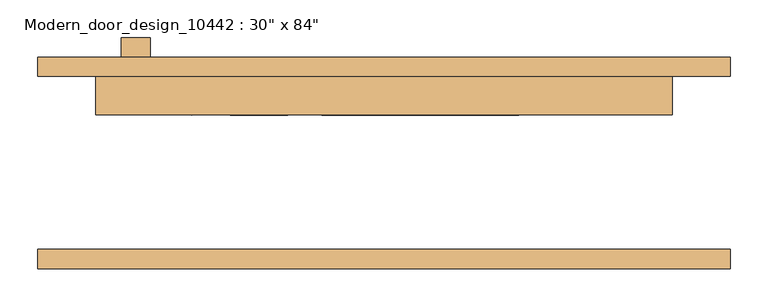
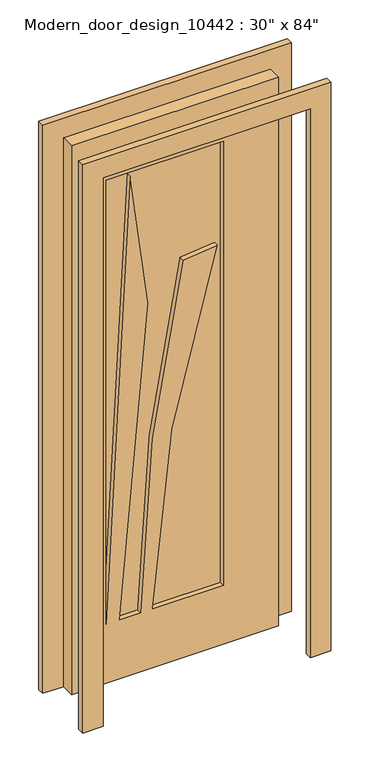
"""IFC4 building model written with IfcOpenShell, lengths in millimetres: door geometry."""

from ifc_helpers import new_model, si_unit, point, frame, frame_2d, origin, place, context, project, spatial, polyline, circle_curve, trimmed, segment, composite_curve, outline, extrude, source, transform, mapped, element, save


def door_beb2f668(model_context):
    return source(origin(), model_context, "Body", "SweptSolid", [
        extrude(outline(composite_curve([segment(polyline([(1955.8, 203.2), (1955.8, -228.6), (228.6, -228.6)]), True, "CONTINUOUS"), segment(trimmed(circle_curve(frame_2d((-685.0101246, 33727.8486678)), 33968.7369443), [point((228.6, -228.6))], [point((1939.1348814, -139.3766773))], True, "CARTESIAN"), True, "CONTINUOUS"), segment(polyline([(1939.1348814, -139.3766773), (1422.9400946, -73.8306519)]), True, "CONTINUOUS"), segment(trimmed(circle_curve(frame_2d((-161.7714181, 11218.4932459)), 11402.9772248), [point((1422.9400946, -73.8306519))], [point((228.6, -177.8))], False, "CARTESIAN"), True, "CONTINUOUS"), segment(polyline([(228.6, -177.8), (228.6, -101.6)]), True, "CONTINUOUS"), segment(trimmed(circle_curve(frame_2d((99.0198331, 6479.552423)), 6582.4279894), [point((228.6, -101.6))], [point((1530.3512301, 54.6284027))], True, "CARTESIAN"), True, "CONTINUOUS"), segment(polyline([(1530.3512301, 54.6284027), (1558.8540137, 182.6647027)]), True, "CONTINUOUS"), segment(trimmed(circle_curve(frame_2d((59.9060717, 4687.9685379)), 4748.1162139), [point((1558.8540137, 182.6647027))], [point((228.6, -57.15))], False, "CARTESIAN"), True, "CONTINUOUS"), segment(polyline([(228.6, -57.15), (228.6, 203.2), (1955.8, 203.2)]), True, "CONTINUOUS")], self_intersect=False)), frame((0.0, 82.55, 0.0), z_axis=(0.0, 1.0, 0.0), x_axis=(0.0, 0.0, 1.0)), (0.0, 0.0, 1.0), 12.7),
        extrude(outline(polyline([(2133.6, 406.4), (2133.6, -355.6), (0.0, -355.6), (0.0, 406.4), (2133.6, 406.4)]), holes=[composite_curve([segment(polyline([(1955.8, 203.2), (228.6, 203.2), (228.6, -57.15)]), True, "CONTINUOUS"), segment(trimmed(circle_curve(frame_2d((59.9060717, 4687.9685379)), 4748.1162139), [point((228.6, -57.15))], [point((1558.8540137, 182.6647027))], True, "CARTESIAN"), True, "CONTINUOUS"), segment(polyline([(1558.8540137, 182.6647027), (1545.3383228, 54.6284027)]), True, "CONTINUOUS"), segment(trimmed(circle_curve(frame_2d((163.0951971, 6077.5340745)), 6179.4812719), [point((1545.3383228, 54.6284027))], [point((228.6, -101.6))], False, "CARTESIAN"), True, "CONTINUOUS"), segment(polyline([(228.6, -101.6), (228.6, -177.8)]), True, "CONTINUOUS"), segment(trimmed(circle_curve(frame_2d((-161.7714181, 11218.4932459)), 11402.9772248), [point((228.6, -177.8))], [point((1422.9400946, -73.8306519))], True, "CARTESIAN"), True, "CONTINUOUS"), segment(polyline([(1422.9400946, -73.8306519), (1939.1348814, -139.3766773)]), True, "CONTINUOUS"), segment(trimmed(circle_curve(frame_2d((-685.0101246, 33727.8486678)), 33968.7369443), [point((1939.1348814, -139.3766773))], [point((228.6, -228.6))], False, "CARTESIAN"), True, "CONTINUOUS"), segment(polyline([(228.6, -228.6), (1955.8, -228.6), (1955.8, 203.2)]), True, "CONTINUOUS")], self_intersect=False)]), frame((0.0, 63.5, 0.0), z_axis=(0.0, 1.0, 0.0), x_axis=(0.0, 0.0, 1.0)), (0.0, 0.0, 1.0), 50.8),
        extrude(outline(polyline([(2209.8, -431.8), (0.0, -431.8), (0.0, -355.6), (2133.6, -355.6), (2133.6, 406.4), (0.0, 406.4), (0.0, 482.6), (2209.8, 482.6), (2209.8, -431.8)])), frame((0.0, 114.3, 0.0), z_axis=(0.0, 1.0, 0.0), x_axis=(0.0, 0.0, 1.0)), (0.0, 0.0, 1.0), 25.4),
        extrude(outline(polyline([(2209.8, 482.6), (2209.8, -431.8), (0.0, -431.8), (0.0, -355.6), (2133.6, -355.6), (2133.6, 406.4), (0.0, 406.4), (0.0, 482.6), (2209.8, 482.6)])), frame((0.0, -139.7, 0.0), z_axis=(0.0, 1.0, 0.0), x_axis=(0.0, 0.0, 1.0)), (0.0, 0.0, 1.0), 25.4),
        extrude(outline(polyline([(-321.6923576, 165.1), (-283.5923576, 165.1), (-283.5923576, 114.3), (-321.6923576, 114.3), (-321.6923576, 165.1)])), frame((0.0, 0.0, 580.9530462), z_axis=(0.0, 0.0, 1.0), x_axis=(1.0, 0.0, 0.0)), (0.0, 0.0, 1.0), 701.7469538),
    ])


if __name__ == "__main__":
    model = new_model("IFC4")
    model_context = context("Model", 3, world=origin())
    ifc_project = project(units=[si_unit("LENGTHUNIT", "METRE", prefix="MILLI")], contexts=[model_context])
    site = spatial("IfcSite", under=ifc_project)
    building = spatial("IfcBuilding", under=site)
    placement = place(None, origin())
    door_shape = door_beb2f668(model_context)
    element("IfcDoor", 1, ObjectType="Modern_door_design_10442 : 30\" x 84\"", at=placement, inside=building, context=model_context, shape_type="MappedRepresentation", body=[
        mapped(door_shape, transform((0.0, 0.0, 0.0), x_axis=(1.0, 0.0, 0.0), y_axis=(0.0, 1.0, 0.0), z_axis=(0.0, 0.0, 1.0))),
    ])
    save(model, "model.ifc")

# Revit data of these elements
# Type "Modern_door_design_10442 : 30\" x 84\""
#   Type Mark = "18"
#   Assembly Code = "C1020"
#   Thickness = 0' - 2"
#   Height = 7' - 0"
#   Muntin = 0' - 1"
#   Stile Width = 0' - 5"
#   Trim Projection Ext = 0' - 1"
#   Trim Projection Int = 0' - 1"
#   Trim Width = 0' - 3"
#   Width = 2' - 6"
#   Door Material = Door - Panel
#   Frame Material = Door - Frame
#   Function = (empty or 0)
#   Wall Closure = (empty or 0)
# Element 1 (IfcDoor, "Modern_door_design_10442 : 30\" x 84\"")
#   Materials on its faces: "Door - Frame", "Door - Panel", "Glass", "Door - Handle"
# Materials
#   "Door - Panel": class "Wood", colour RGB 210 159 95, transparency 0, Cost = 0
#   "Door - Frame": colour RGB 118 70 51, transparency 0, Cost = 0
#   "Glass": class "Glass", colour RGB 0 128 192, transparency 0.75, Description = "Soda Lime Glass", Cost = 0
#   "Door - Handle": class "Metal", colour RGB 164 185 197, transparency 0
